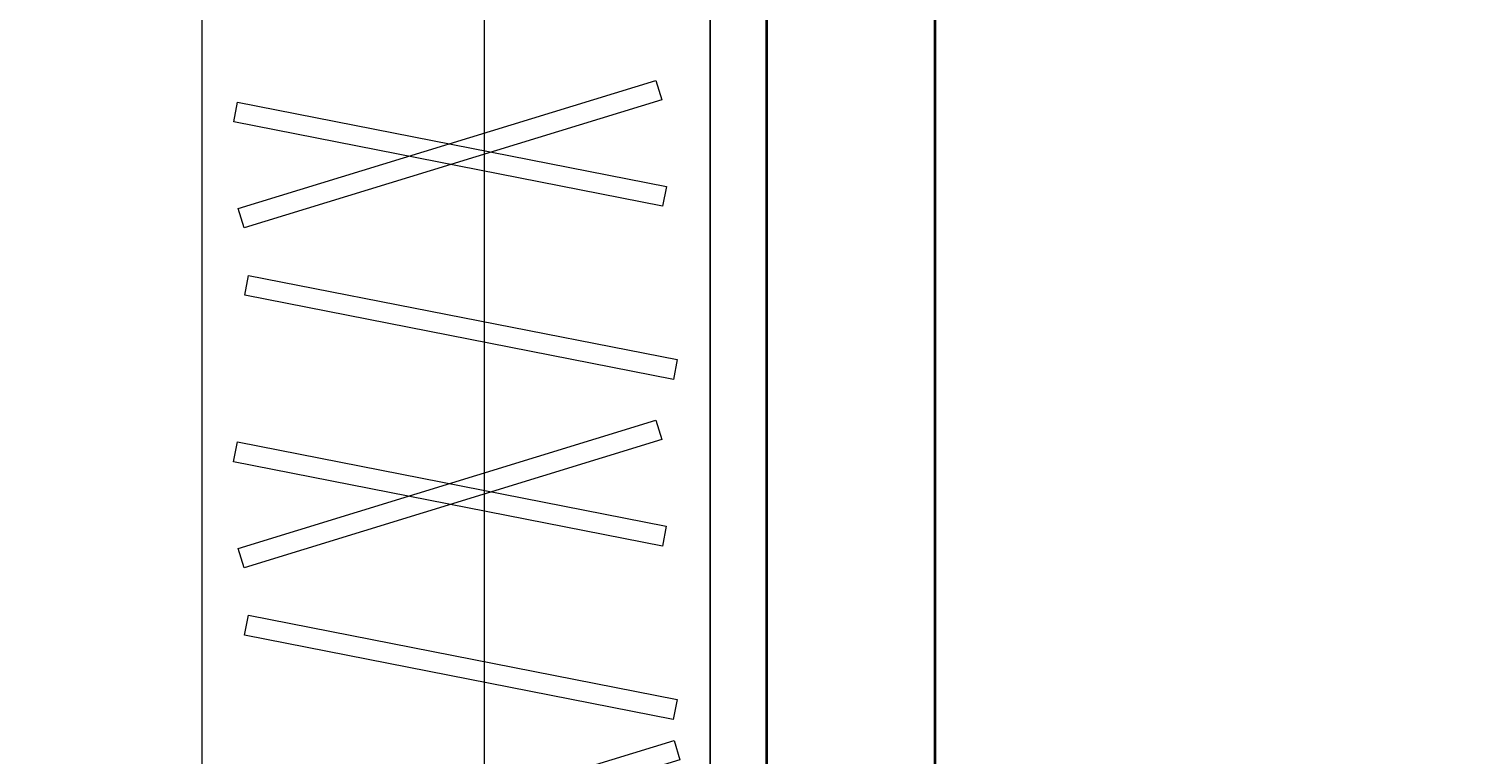
# Model space of a CAD drawing. Units: inches. Extents: x -61 to 1599, y -1316 to 257.
# Tile 69 of 204: x 295 to 347, y -680 to -654. Entities that reach past the tile are written whole.
import ezdxf

# ---------------------------------------------------------------- set-up
doc = ezdxf.new("R2010")
doc.units = ezdxf.units.IN
doc.header["$MEASUREMENT"] = 0
for name, color, linetype, lineweight in [('A-ANNO-DIMS', 2, 'Continuous', 18), ('A-FLOR-CASE', 8, 'Continuous', 18), ('WALLS', 4, 'Continuous', 35)]:
    doc.layers.add(name, color=color, linetype=linetype, lineweight=lineweight)
doc.styles.get("Standard").update_dxf_attribs({"font": 'arial.ttf'})
doc.dimstyles.get("Standard").update_dxf_attribs({"dimtxt": 0.18, "dimasz": 0.18, "dimexe": 0.18, "dimexo": 0.0625, "dimgap": 0.09, "dimtad": 0, "dimtih": 1, "dimtoh": 1, "dimdec": 0, "dimzin": 0, "dimdsep": 46, "dimlunit": 3, "dimtxsty": 'Standard', "dimcen": 0.09, "dimadec": 0, "dimazin": 0, "dimtfac": 1, "dimtdec": 0, "dimtofl": 0, "dimtmove": 0, "dimatfit": 3, "dimfxl": 1, "dimtolj": 1, "dimtzin": 0, "dimarcsym": 0})

# ---------------------------------------------------------------- blocks, each defined once
blk = doc.blocks.new('WARDROBE-HANGING')
blk.add_line((10.047, 0), (10.047, 68))
for points in [[(20.094, 0), (0, 0), (0, 68), (20.094, 68)], [(1.283, 33.408), (16.158, 37.977), (16.37, 37.289), (1.495, 32.72)], [(1.262, 37.203), (16.53, 34.2), (16.391, 33.493), (1.123, 36.497)], [(1.651, 31.03), (16.919, 28.027), (16.78, 27.32), (1.512, 30.324)], [(1.279, 21.299), (16.154, 25.868), (16.365, 25.18), (1.49, 20.611)], [(1.257, 25.094), (16.525, 22.091), (16.386, 21.384), (1.118, 24.388)], [(1.646, 18.921), (16.914, 15.918), (16.775, 15.211), (1.507, 18.215)], [(1.928, 9.892), (16.803, 14.461), (17.014, 13.773), (2.139, 9.203)]]:
    blk.add_lwpolyline(points, close=True)
blk = doc.blocks.new('*D687')
at = {"layer": 'A-ANNO-DIMS', "color": 0, "lineweight": -2, "transparency": 16777216}
for p, q in [((289.418, 181.677), (-61.077, 181.677)), ((-60.897, 181.497), (-60.897, -528.952)), ((-60.897, -1239.765), (-60.897, -529.316)), ((319.64, -1239.945), (-61.077, -1239.945))]:
    blk.add_line(p, q, dxfattribs=at)
at = {"layer": 'A-ANNO-DIMS', "color": 0, "transparency": 16777216}
for points in [[(-60.927, 181.497), (-60.867, 181.497), (-60.897, 181.677)], [(-60.927, -1239.765), (-60.867, -1239.765), (-60.897, -1239.945)]]:
    blk.add_solid(points, dxfattribs=at)
at = {"layer": 'DEFPOINTS', "color": 0, "transparency": 16777216}
for p in [(289.481, 181.677), (-60.897, -1239.945), (319.703, -1239.945)]:
    blk.add_point(p, dxfattribs=at)
at = {"layer": 'A-ANNO-DIMS', "color": 0, "transparency": 16777216, "insert": (-60.897, -529.134), "char_height": 0.18, "attachment_point": 5}
blk.add_mtext('\\A1;1421.6', dxfattribs=at)
blk = doc.blocks.new('*D710')
at = {"layer": 'A-ANNO-DIMS', "color": 0, "lineweight": -2, "transparency": 16777216}
for p, q in [((319.703, -465.385), (319.703, -1315.725)), ((403.703, -465.385), (403.703, -1315.725)), ((319.883, -1315.545), (361.484, -1315.545)), ((403.523, -1315.545), (361.921, -1315.545))]:
    blk.add_line(p, q, dxfattribs=at)
at = {"layer": 'A-ANNO-DIMS', "color": 0, "transparency": 16777216}
for points in [[(319.883, -1315.515), (319.883, -1315.575), (319.703, -1315.545)], [(403.523, -1315.515), (403.523, -1315.575), (403.703, -1315.545)]]:
    blk.add_solid(points, dxfattribs=at)
at = {"layer": 'DEFPOINTS', "color": 0, "transparency": 16777216}
for p in [(319.703, -465.323), (403.703, -465.323), (403.703, -1315.545)]:
    blk.add_point(p, dxfattribs=at)
at = {"layer": 'A-ANNO-DIMS', "color": 0, "transparency": 16777216, "insert": (361.703, -1315.545), "char_height": 0.18, "attachment_point": 5}
blk.add_mtext('\\A1;84', dxfattribs=at)

msp = doc.modelspace()

# ---------------------------------------------------------------- linework, layer by layer
at = {"layer": 'WALLS'}
for p, q in [((321.7028, -616.9446), (321.7028, -787.9446)), ((327.7028, -616.9446), (327.7028, -787.9446))]:
    msp.add_line(p, q, dxfattribs=at)

# ---------------------------------------------------------------- block references
at = {"layer": 'A-FLOR-CASE'}
msp.add_blockref('WARDROBE-HANGING', (301.609, -693.9447), dxfattribs=at)

# ---------------------------------------------------------------- dimensions: what is measured, and where the dimension line sits
at = {"layer": 'A-ANNO-DIMS'}
dim = msp.add_linear_dim(base=(-60.8972, -1239.9446), p1=(289.4807, 181.6771), p2=(319.7028, -1239.9446), angle=90, dimstyle='Standard', override={"dimdec": 1, "dimlfac": 1, "dimrnd": 0, "dimzin": 0, "dimdsep": 46, "dimlunit": 2}, dxfattribs=at)
dim.commit()
dim.dimension.update_dxf_attribs({"geometry": '*D687', "text_midpoint": (-60.8972, -529.1337)})
dim = msp.add_linear_dim(base=(403.7028, -1315.5446), p1=(319.7028, -465.3229), p2=(403.7028, -465.3229), dimstyle='Standard', override={"dimdec": 0, "dimlfac": 1, "dimrnd": 0, "dimzin": 0, "dimdsep": 46, "dimlunit": 2}, dxfattribs=at)
dim.commit()
dim.dimension.update_dxf_attribs({"geometry": '*D710', "text_midpoint": (361.7028, -1315.5446)})

doc.saveas('drawing.dxf')
